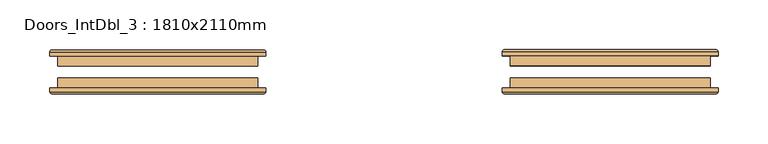
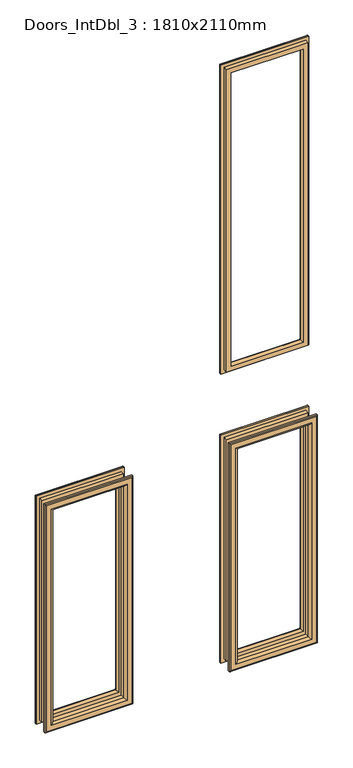
"""IFC4 building model written with IfcOpenShell, lengths in millimetres: door geometry, Doors_IntDbl_3 : 1810x2110mm."""

from ifc_helpers import new_model, si_unit, frame, origin, place, context, project, spatial, ellipse_curve, source, transform, mapped, element, save
from ifc_brep_helpers import plane_surface, cylinder_surface, advanced_brep


def doors_intdbl_3_1810x2110mm_13513f6f(model_context):
    return source(origin(), model_context, "Body", "AdvancedBrep", [
        advanced_brep(
        [(326.5, -79.6, 1885.0), (326.5, -79.6, 1100.0), (326.5, -69.6, 1100.0), (326.5, -69.6, 1885.0), (314.5, -68.6, 1873.0), (314.5, -68.6, 1112.0), (314.5, -79.6, 1112.0), (314.5, -79.6, 1873.0), (319.5, -63.6, 1878.0), (319.5, -63.6, 1107.0), (334.5, -65.6, 1893.0), (334.5, -65.6, 1092.0), (332.5, -63.6, 1094.0), (332.5, -63.6, 1891.0), (334.5, -69.6, 1893.0), (334.5, -69.6, 1092.0), (126.5, -79.6, 1100.0), (126.5, -69.6, 1100.0), (138.5, -68.6, 1112.0), (138.5, -79.6, 1112.0), (133.5, -63.6, 1107.0), (118.5, -65.6, 1092.0), (120.5, -63.6, 1094.0), (118.5, -69.6, 1092.0), (126.5, -79.6, 1885.0), (126.5, -69.6, 1885.0), (138.5, -68.6, 1873.0), (138.5, -79.6, 1873.0), (133.5, -63.6, 1878.0), (118.5, -65.6, 1893.0), (120.5, -63.6, 1891.0), (118.5, -69.6, 1893.0)],
        [
            (0, 1),
            (1, 2),
            (2, 3),
            (3, 0),
            (4, 5),
            (5, 6),
            (6, 7),
            (7, 4),
            (8, 9),
            (9, 5, ellipse_curve(frame((319.5, -68.6, 1107.0), z_axis=(0.7071067811865475, 0.0, 0.7071067811865475), x_axis=(-0.7071067811865474, 0.0, 0.7071067811865476)), 7.0710678, 5.0)),
            (4, 8, ellipse_curve(frame((319.5, -68.6, 1878.0), z_axis=(0.7071067811865475, 0.0, -0.7071067811865475), x_axis=(0.7071067811865474, 0.0, 0.7071067811865476)), 7.0710678, 5.0)),
            (10, 11),
            (11, 12, ellipse_curve(frame((332.5, -65.6, 1094.0), z_axis=(0.7071067811865475, 0.0, 0.7071067811865475), x_axis=(-0.7071067811865474, 0.0, 0.7071067811865476)), 2.8284271, 2.0)),
            (12, 13),
            (13, 10, ellipse_curve(frame((332.5, -65.6, 1891.0), z_axis=(0.7071067811865475, 0.0, -0.7071067811865475), x_axis=(0.7071067811865474, 0.0, 0.7071067811865476)), 2.8284271, 2.0)),
            (14, 15),
            (15, 11),
            (10, 14),
            (1, 16),
            (16, 17),
            (17, 2),
            (5, 18),
            (18, 19),
            (19, 6),
            (9, 20),
            (20, 18, ellipse_curve(frame((133.5, -68.6, 1107.0), z_axis=(0.7071067811865475, 0.0, -0.7071067811865475), x_axis=(0.7071067811865476, 0.0, 0.7071067811865474)), 7.0710678, 5.0)),
            (11, 21),
            (21, 22, ellipse_curve(frame((120.5, -65.6, 1094.0), z_axis=(0.7071067811865475, 0.0, -0.7071067811865475), x_axis=(0.7071067811865476, 0.0, 0.7071067811865474)), 2.8284271, 2.0)),
            (22, 12),
            (15, 23),
            (23, 21),
            (16, 24),
            (24, 25),
            (25, 17),
            (18, 26),
            (26, 27),
            (27, 19),
            (20, 28),
            (28, 26, ellipse_curve(frame((133.5, -68.6, 1878.0), z_axis=(-0.7071067811865475, 0.0, -0.7071067811865475), x_axis=(0.7071067811865474, 0.0, -0.7071067811865476)), 7.0710678, 5.0)),
            (21, 29),
            (29, 30, ellipse_curve(frame((120.5, -65.6, 1891.0), z_axis=(-0.7071067811865475, 0.0, -0.7071067811865475), x_axis=(0.7071067811865474, 0.0, -0.7071067811865476)), 2.8284271, 2.0)),
            (30, 22),
            (23, 31),
            (31, 29),
            (14, 31),
            (25, 3),
            (24, 0),
            (27, 7),
            (26, 4),
            (28, 8),
            (30, 13),
            (29, 10),
        ],
        [
            plane_surface(frame((326.5, -69.6, 1885.0), z_axis=(1.0, 0.0, 0.0), x_axis=(0.0, 0.0, -1.0))),
            plane_surface(frame((314.5, -79.6, 1873.0), z_axis=(-1.0, 0.0, 0.0), x_axis=(0.0, 0.0, -1.0))),
            cylinder_surface(frame((319.5, -68.6, 1885.0), z_axis=(0.0, 0.0, 1.0), x_axis=(1.0, 0.0, 0.0)), 5.0),
            cylinder_surface(frame((332.5, -65.6, 1885.0), z_axis=(0.0, 0.0, 1.0), x_axis=(1.0, 0.0, 0.0)), 2.0),
            plane_surface(frame((334.5, -65.6, 1893.0), z_axis=(1.0, 0.0, 0.0), x_axis=(0.0, 0.0, -1.0))),
            plane_surface(frame((326.5, -69.6, 1100.0), z_axis=(0.0, 0.0, -1.0), x_axis=(-1.0, 0.0, 0.0))),
            plane_surface(frame((314.5, -79.6, 1112.0), z_axis=(0.0, 0.0, 1.0), x_axis=(-1.0, 0.0, 0.0))),
            cylinder_surface(frame((326.5, -68.6, 1107.0), z_axis=(1.0, 0.0, 0.0), x_axis=(0.0, 0.0, -1.0)), 5.0),
            cylinder_surface(frame((326.5, -65.6, 1094.0), z_axis=(1.0, 0.0, 0.0), x_axis=(0.0, 0.0, -1.0)), 2.0),
            plane_surface(frame((334.5, -65.6, 1092.0), z_axis=(0.0, 0.0, -1.0), x_axis=(-1.0, 0.0, 0.0))),
            plane_surface(frame((126.5, -69.6, 1100.0), z_axis=(-1.0, 0.0, 0.0), x_axis=(0.0, 0.0, 1.0))),
            plane_surface(frame((138.5, -79.6, 1112.0), z_axis=(1.0, 0.0, 0.0), x_axis=(0.0, 0.0, 1.0))),
            cylinder_surface(frame((133.5, -68.6, 1100.0), z_axis=(0.0, 0.0, -1.0), x_axis=(-1.0, 0.0, 0.0)), 5.0),
            cylinder_surface(frame((120.5, -65.6, 1100.0), z_axis=(0.0, 0.0, -1.0), x_axis=(-1.0, 0.0, 0.0)), 2.0),
            plane_surface(frame((118.5, -65.6, 1092.0), z_axis=(-1.0, 0.0, 0.0), x_axis=(0.0, 0.0, 1.0))),
            plane_surface(frame((118.5, -69.6, 1893.0), z_axis=(0.0, -1.0, 0.0), x_axis=(1.0, 0.0, 0.0))),
            plane_surface(frame((126.5, -69.6, 1885.0), z_axis=(0.0, 0.0, 1.0), x_axis=(1.0, 0.0, 0.0))),
            plane_surface(frame((126.5, -79.6, 1885.0), z_axis=(0.0, -1.0, 0.0), x_axis=(1.0, 0.0, 0.0))),
            plane_surface(frame((138.5, -79.6, 1873.0), z_axis=(0.0, 0.0, -1.0), x_axis=(1.0, 0.0, 0.0))),
            cylinder_surface(frame((126.5, -68.6, 1878.0), z_axis=(-1.0, 0.0, 0.0), x_axis=(0.0, 0.0, 1.0)), 5.0),
            plane_surface(frame((133.5, -63.6, 1878.0), z_axis=(0.0, 1.0, 0.0), x_axis=(1.0, 0.0, 0.0))),
            cylinder_surface(frame((126.5, -65.6, 1891.0), z_axis=(-1.0, 0.0, 0.0), x_axis=(0.0, 0.0, 1.0)), 2.0),
            plane_surface(frame((118.5, -65.6, 1893.0), z_axis=(0.0, 0.0, 1.0), x_axis=(1.0, 0.0, 0.0))),
        ],
        [
            (0, [[1, 2, 3, 4]]),
            (1, [[5, 6, 7, 8]]),
            (2, [[9, 10, -5, 11]]),
            (3, [[12, 13, 14, 15]]),
            (4, [[16, 17, -12, 18]]),
            (5, [[19, 20, 21, -2]]),
            (6, [[22, 23, 24, -6]]),
            (7, [[25, 26, -22, -10]]),
            (8, [[27, 28, 29, -13]]),
            (9, [[30, 31, -27, -17]]),
            (10, [[32, 33, 34, -20]]),
            (11, [[35, 36, 37, -23]]),
            (12, [[38, 39, -35, -26]]),
            (13, [[40, 41, 42, -28]]),
            (14, [[43, 44, -40, -31]]),
            (15, [[-16, 45, -43, -30], [-3, -21, -34, 46]]),
            (16, [[47, -4, -46, -33]]),
            (17, [[-1, -47, -32, -19], [-7, -24, -37, 48]]),
            (18, [[49, -8, -48, -36]]),
            (19, [[50, -11, -49, -39]]),
            (20, [[-14, -29, -42, 51], [-9, -50, -38, -25]]),
            (21, [[52, -15, -51, -41]]),
            (22, [[-45, -18, -52, -44]]),
        ],
    ),
        advanced_brep(
        [(118.5, -105.6, 342.0), (118.5, -105.6, 933.0), (118.5, -101.6, 933.0), (118.5, -101.6, 342.0), (120.5, -107.6, 344.0), (120.5, -107.6, 931.0), (138.5, -102.6, 362.0), (138.5, -102.6, 913.0), (133.5, -107.6, 918.0), (133.5, -107.6, 357.0), (138.5, -91.6, 362.0), (138.5, -91.6, 913.0), (126.5, -101.6, 350.0), (126.5, -101.6, 925.0), (126.5, -91.6, 925.0), (126.5, -91.6, 350.0), (334.5, -105.6, 933.0), (334.5, -101.6, 933.0), (332.5, -107.6, 931.0), (314.5, -102.6, 913.0), (319.5, -107.6, 918.0), (314.5, -91.6, 913.0), (326.5, -101.6, 925.0), (326.5, -91.6, 925.0), (334.5, -105.6, 342.0), (334.5, -101.6, 342.0), (332.5, -107.6, 344.0), (314.5, -102.6, 362.0), (319.5, -107.6, 357.0), (314.5, -91.6, 362.0), (326.5, -101.6, 350.0), (326.5, -91.6, 350.0)],
        [
            (0, 1),
            (1, 2),
            (2, 3),
            (3, 0),
            (4, 5),
            (5, 1, ellipse_curve(frame((120.5, -105.6, 931.0), z_axis=(-0.7071067811865475, 0.0, -0.7071067811865475), x_axis=(0.7071067811865474, 0.0, -0.7071067811865476)), 2.8284271, 2.0)),
            (0, 4, ellipse_curve(frame((120.5, -105.6, 344.0), z_axis=(-0.7071067811865475, 0.0, 0.7071067811865475), x_axis=(-0.7071067811865474, 0.0, -0.7071067811865476)), 2.8284271, 2.0)),
            (6, 7),
            (7, 8, ellipse_curve(frame((133.5, -102.6, 918.0), z_axis=(-0.7071067811865475, 0.0, -0.7071067811865475), x_axis=(0.7071067811865474, 0.0, -0.7071067811865476)), 7.0710678, 5.0)),
            (8, 9),
            (9, 6, ellipse_curve(frame((133.5, -102.6, 357.0), z_axis=(-0.7071067811865475, 0.0, 0.7071067811865475), x_axis=(-0.7071067811865474, 0.0, -0.7071067811865476)), 7.0710678, 5.0)),
            (10, 11),
            (11, 7),
            (6, 10),
            (12, 13),
            (13, 14),
            (14, 15),
            (15, 12),
            (1, 16),
            (16, 17),
            (17, 2),
            (5, 18),
            (18, 16, ellipse_curve(frame((332.5, -105.6, 931.0), z_axis=(-0.7071067811865475, 0.0, 0.7071067811865475), x_axis=(-0.7071067811865476, 0.0, -0.7071067811865474)), 2.8284271, 2.0)),
            (7, 19),
            (19, 20, ellipse_curve(frame((319.5, -102.6, 918.0), z_axis=(-0.7071067811865475, 0.0, 0.7071067811865475), x_axis=(-0.7071067811865476, 0.0, -0.7071067811865474)), 7.0710678, 5.0)),
            (20, 8),
            (11, 21),
            (21, 19),
            (13, 22),
            (22, 23),
            (23, 14),
            (16, 24),
            (24, 25),
            (25, 17),
            (18, 26),
            (26, 24, ellipse_curve(frame((332.5, -105.6, 344.0), z_axis=(0.7071067811865475, 0.0, 0.7071067811865475), x_axis=(-0.7071067811865474, 0.0, 0.7071067811865476)), 2.8284271, 2.0)),
            (19, 27),
            (27, 28, ellipse_curve(frame((319.5, -102.6, 357.0), z_axis=(0.7071067811865475, 0.0, 0.7071067811865475), x_axis=(-0.7071067811865474, 0.0, 0.7071067811865476)), 7.0710678, 5.0)),
            (28, 20),
            (21, 29),
            (29, 27),
            (22, 30),
            (30, 31),
            (31, 23),
            (24, 0),
            (3, 25),
            (26, 4),
            (28, 9),
            (27, 6),
            (29, 10),
            (31, 15),
            (30, 12),
        ],
        [
            plane_surface(frame((118.5, -101.6, 342.0), z_axis=(-1.0, 0.0, 0.0), x_axis=(0.0, 0.0, 1.0))),
            cylinder_surface(frame((120.5, -105.6, 350.0), z_axis=(0.0, 0.0, -1.0), x_axis=(-1.0, 0.0, 0.0)), 2.0),
            cylinder_surface(frame((133.5, -102.6, 350.0), z_axis=(0.0, 0.0, -1.0), x_axis=(-1.0, 0.0, 0.0)), 5.0),
            plane_surface(frame((138.5, -102.6, 362.0), z_axis=(1.0, 0.0, 0.0), x_axis=(0.0, 0.0, 1.0))),
            plane_surface(frame((126.5, -91.6, 350.0), z_axis=(-1.0, 0.0, 0.0), x_axis=(0.0, 0.0, 1.0))),
            plane_surface(frame((118.5, -101.6, 933.0), z_axis=(0.0, 0.0, 1.0), x_axis=(1.0, 0.0, 0.0))),
            cylinder_surface(frame((126.5, -105.6, 931.0), z_axis=(-1.0, 0.0, 0.0), x_axis=(0.0, 0.0, 1.0)), 2.0),
            cylinder_surface(frame((126.5, -102.6, 918.0), z_axis=(-1.0, 0.0, 0.0), x_axis=(0.0, 0.0, 1.0)), 5.0),
            plane_surface(frame((138.5, -102.6, 913.0), z_axis=(0.0, 0.0, -1.0), x_axis=(1.0, 0.0, 0.0))),
            plane_surface(frame((126.5, -91.6, 925.0), z_axis=(0.0, 0.0, 1.0), x_axis=(1.0, 0.0, 0.0))),
            plane_surface(frame((334.5, -101.6, 933.0), z_axis=(1.0, 0.0, 0.0), x_axis=(0.0, 0.0, -1.0))),
            cylinder_surface(frame((332.5, -105.6, 925.0), z_axis=(0.0, 0.0, 1.0), x_axis=(1.0, 0.0, 0.0)), 2.0),
            cylinder_surface(frame((319.5, -102.6, 925.0), z_axis=(0.0, 0.0, 1.0), x_axis=(1.0, 0.0, 0.0)), 5.0),
            plane_surface(frame((314.5, -102.6, 913.0), z_axis=(-1.0, 0.0, 0.0), x_axis=(0.0, 0.0, -1.0))),
            plane_surface(frame((326.5, -91.6, 925.0), z_axis=(1.0, 0.0, 0.0), x_axis=(0.0, 0.0, -1.0))),
            plane_surface(frame((334.5, -101.6, 342.0), z_axis=(0.0, 0.0, -1.0), x_axis=(-1.0, 0.0, 0.0))),
            cylinder_surface(frame((326.5, -105.6, 344.0), z_axis=(1.0, 0.0, 0.0), x_axis=(0.0, 0.0, -1.0)), 2.0),
            plane_surface(frame((332.5, -107.6, 344.0), z_axis=(0.0, -1.0, 0.0), x_axis=(-1.0, 0.0, 0.0))),
            cylinder_surface(frame((326.5, -102.6, 357.0), z_axis=(1.0, 0.0, 0.0), x_axis=(0.0, 0.0, -1.0)), 5.0),
            plane_surface(frame((314.5, -102.6, 362.0), z_axis=(0.0, 0.0, 1.0), x_axis=(-1.0, 0.0, 0.0))),
            plane_surface(frame((314.5, -91.6, 362.0), z_axis=(0.0, 1.0, 0.0), x_axis=(-1.0, 0.0, 0.0))),
            plane_surface(frame((326.5, -91.6, 350.0), z_axis=(0.0, 0.0, -1.0), x_axis=(-1.0, 0.0, 0.0))),
            plane_surface(frame((326.5, -101.6, 350.0), z_axis=(0.0, 1.0, 0.0), x_axis=(-1.0, 0.0, 0.0))),
        ],
        [
            (0, [[1, 2, 3, 4]]),
            (1, [[5, 6, -1, 7]]),
            (2, [[8, 9, 10, 11]]),
            (3, [[12, 13, -8, 14]]),
            (4, [[15, 16, 17, 18]]),
            (5, [[19, 20, 21, -2]]),
            (6, [[22, 23, -19, -6]]),
            (7, [[24, 25, 26, -9]]),
            (8, [[27, 28, -24, -13]]),
            (9, [[29, 30, 31, -16]]),
            (10, [[32, 33, 34, -20]]),
            (11, [[35, 36, -32, -23]]),
            (12, [[37, 38, 39, -25]]),
            (13, [[40, 41, -37, -28]]),
            (14, [[42, 43, 44, -30]]),
            (15, [[45, -4, 46, -33]]),
            (16, [[47, -7, -45, -36]]),
            (17, [[-5, -47, -35, -22], [-10, -26, -39, 48]]),
            (18, [[49, -11, -48, -38]]),
            (19, [[50, -14, -49, -41]]),
            (20, [[-17, -31, -44, 51], [-12, -50, -40, -27]]),
            (21, [[52, -18, -51, -43]]),
            (22, [[-3, -21, -34, -46], [-15, -52, -42, -29]]),
        ],
    ),
        advanced_brep(
        [(-334.5, -105.6, 342.0), (-334.5, -105.6, 933.0), (-334.5, -101.6, 933.0), (-334.5, -101.6, 342.0), (-332.5, -107.6, 344.0), (-332.5, -107.6, 931.0), (-314.5, -102.6, 362.0), (-314.5, -102.6, 913.0), (-319.5, -107.6, 918.0), (-319.5, -107.6, 357.0), (-314.5, -91.6, 362.0), (-314.5, -91.6, 913.0), (-326.5, -101.6, 350.0), (-326.5, -101.6, 925.0), (-326.5, -91.6, 925.0), (-326.5, -91.6, 350.0), (-118.5, -105.6, 933.0), (-118.5, -101.6, 933.0), (-120.5, -107.6, 931.0), (-138.5, -102.6, 913.0), (-133.5, -107.6, 918.0), (-138.5, -91.6, 913.0), (-126.5, -101.6, 925.0), (-126.5, -91.6, 925.0), (-118.5, -105.6, 342.0), (-118.5, -101.6, 342.0), (-120.5, -107.6, 344.0), (-138.5, -102.6, 362.0), (-133.5, -107.6, 357.0), (-138.5, -91.6, 362.0), (-126.5, -101.6, 350.0), (-126.5, -91.6, 350.0)],
        [
            (0, 1),
            (1, 2),
            (2, 3),
            (3, 0),
            (4, 5),
            (5, 1, ellipse_curve(frame((-332.5, -105.6, 931.0), z_axis=(-0.7071067811865475, 0.0, -0.7071067811865475), x_axis=(0.7071067811865474, 0.0, -0.7071067811865476)), 2.8284271, 2.0)),
            (0, 4, ellipse_curve(frame((-332.5, -105.6, 344.0), z_axis=(-0.7071067811865475, 0.0, 0.7071067811865475), x_axis=(-0.7071067811865474, 0.0, -0.7071067811865476)), 2.8284271, 2.0)),
            (6, 7),
            (7, 8, ellipse_curve(frame((-319.5, -102.6, 918.0), z_axis=(-0.7071067811865475, 0.0, -0.7071067811865475), x_axis=(0.7071067811865474, 0.0, -0.7071067811865476)), 7.0710678, 5.0)),
            (8, 9),
            (9, 6, ellipse_curve(frame((-319.5, -102.6, 357.0), z_axis=(-0.7071067811865475, 0.0, 0.7071067811865475), x_axis=(-0.7071067811865474, 0.0, -0.7071067811865476)), 7.0710678, 5.0)),
            (10, 11),
            (11, 7),
            (6, 10),
            (12, 13),
            (13, 14),
            (14, 15),
            (15, 12),
            (1, 16),
            (16, 17),
            (17, 2),
            (5, 18),
            (18, 16, ellipse_curve(frame((-120.5, -105.6, 931.0), z_axis=(-0.7071067811865475, 0.0, 0.7071067811865475), x_axis=(-0.7071067811865476, 0.0, -0.7071067811865474)), 2.8284271, 2.0)),
            (7, 19),
            (19, 20, ellipse_curve(frame((-133.5, -102.6, 918.0), z_axis=(-0.7071067811865475, 0.0, 0.7071067811865475), x_axis=(-0.7071067811865476, 0.0, -0.7071067811865474)), 7.0710678, 5.0)),
            (20, 8),
            (11, 21),
            (21, 19),
            (13, 22),
            (22, 23),
            (23, 14),
            (16, 24),
            (24, 25),
            (25, 17),
            (18, 26),
            (26, 24, ellipse_curve(frame((-120.5, -105.6, 344.0), z_axis=(0.7071067811865475, 0.0, 0.7071067811865475), x_axis=(-0.7071067811865474, 0.0, 0.7071067811865476)), 2.8284271, 2.0)),
            (19, 27),
            (27, 28, ellipse_curve(frame((-133.5, -102.6, 357.0), z_axis=(0.7071067811865475, 0.0, 0.7071067811865475), x_axis=(-0.7071067811865474, 0.0, 0.7071067811865476)), 7.0710678, 5.0)),
            (28, 20),
            (21, 29),
            (29, 27),
            (22, 30),
            (30, 31),
            (31, 23),
            (24, 0),
            (3, 25),
            (26, 4),
            (28, 9),
            (27, 6),
            (29, 10),
            (31, 15),
            (30, 12),
        ],
        [
            plane_surface(frame((-334.5, -101.6, 342.0), z_axis=(-1.0, 0.0, 0.0), x_axis=(0.0, 0.0, 1.0))),
            cylinder_surface(frame((-332.5, -105.6, 350.0), z_axis=(0.0, 0.0, -1.0), x_axis=(-1.0, 0.0, 0.0)), 2.0),
            cylinder_surface(frame((-319.5, -102.6, 350.0), z_axis=(0.0, 0.0, -1.0), x_axis=(-1.0, 0.0, 0.0)), 5.0),
            plane_surface(frame((-314.5, -102.6, 362.0), z_axis=(1.0, 0.0, 0.0), x_axis=(0.0, 0.0, 1.0))),
            plane_surface(frame((-326.5, -91.6, 350.0), z_axis=(-1.0, 0.0, 0.0), x_axis=(0.0, 0.0, 1.0))),
            plane_surface(frame((-334.5, -101.6, 933.0), z_axis=(0.0, 0.0, 1.0), x_axis=(1.0, 0.0, 0.0))),
            cylinder_surface(frame((-326.5, -105.6, 931.0), z_axis=(-1.0, 0.0, 0.0), x_axis=(0.0, 0.0, 1.0)), 2.0),
            cylinder_surface(frame((-326.5, -102.6, 918.0), z_axis=(-1.0, 0.0, 0.0), x_axis=(0.0, 0.0, 1.0)), 5.0),
            plane_surface(frame((-314.5, -102.6, 913.0), z_axis=(0.0, 0.0, -1.0), x_axis=(1.0, 0.0, 0.0))),
            plane_surface(frame((-326.5, -91.6, 925.0), z_axis=(0.0, 0.0, 1.0), x_axis=(1.0, 0.0, 0.0))),
            plane_surface(frame((-118.5, -101.6, 933.0), z_axis=(1.0, 0.0, 0.0), x_axis=(0.0, 0.0, -1.0))),
            cylinder_surface(frame((-120.5, -105.6, 925.0), z_axis=(0.0, 0.0, 1.0), x_axis=(1.0, 0.0, 0.0)), 2.0),
            cylinder_surface(frame((-133.5, -102.6, 925.0), z_axis=(0.0, 0.0, 1.0), x_axis=(1.0, 0.0, 0.0)), 5.0),
            plane_surface(frame((-138.5, -102.6, 913.0), z_axis=(-1.0, 0.0, 0.0), x_axis=(0.0, 0.0, -1.0))),
            plane_surface(frame((-126.5, -91.6, 925.0), z_axis=(1.0, 0.0, 0.0), x_axis=(0.0, 0.0, -1.0))),
            plane_surface(frame((-118.5, -101.6, 342.0), z_axis=(0.0, 0.0, -1.0), x_axis=(-1.0, 0.0, 0.0))),
            cylinder_surface(frame((-126.5, -105.6, 344.0), z_axis=(1.0, 0.0, 0.0), x_axis=(0.0, 0.0, -1.0)), 2.0),
            plane_surface(frame((-120.5, -107.6, 344.0), z_axis=(0.0, -1.0, 0.0), x_axis=(-1.0, 0.0, 0.0))),
            cylinder_surface(frame((-126.5, -102.6, 357.0), z_axis=(1.0, 0.0, 0.0), x_axis=(0.0, 0.0, -1.0)), 5.0),
            plane_surface(frame((-138.5, -102.6, 362.0), z_axis=(0.0, 0.0, 1.0), x_axis=(-1.0, 0.0, 0.0))),
            plane_surface(frame((-138.5, -91.6, 362.0), z_axis=(0.0, 1.0, 0.0), x_axis=(-1.0, 0.0, 0.0))),
            plane_surface(frame((-126.5, -91.6, 350.0), z_axis=(0.0, 0.0, -1.0), x_axis=(-1.0, 0.0, 0.0))),
            plane_surface(frame((-126.5, -101.6, 350.0), z_axis=(0.0, 1.0, 0.0), x_axis=(-1.0, 0.0, 0.0))),
        ],
        [
            (0, [[1, 2, 3, 4]]),
            (1, [[5, 6, -1, 7]]),
            (2, [[8, 9, 10, 11]]),
            (3, [[12, 13, -8, 14]]),
            (4, [[15, 16, 17, 18]]),
            (5, [[19, 20, 21, -2]]),
            (6, [[22, 23, -19, -6]]),
            (7, [[24, 25, 26, -9]]),
            (8, [[27, 28, -24, -13]]),
            (9, [[29, 30, 31, -16]]),
            (10, [[32, 33, 34, -20]]),
            (11, [[35, 36, -32, -23]]),
            (12, [[37, 38, 39, -25]]),
            (13, [[40, 41, -37, -28]]),
            (14, [[42, 43, 44, -30]]),
            (15, [[45, -4, 46, -33]]),
            (16, [[47, -7, -45, -36]]),
            (17, [[-5, -47, -35, -22], [-10, -26, -39, 48]]),
            (18, [[49, -11, -48, -38]]),
            (19, [[50, -14, -49, -41]]),
            (20, [[-17, -31, -44, 51], [-12, -50, -40, -27]]),
            (21, [[52, -18, -51, -43]]),
            (22, [[-3, -21, -34, -46], [-15, -52, -42, -29]]),
        ],
    ),
        advanced_brep(
        [(-126.5, -79.6, 925.0), (-126.5, -79.6, 350.0), (-126.5, -69.6, 350.0), (-126.5, -69.6, 925.0), (-138.5, -68.6, 913.0), (-138.5, -68.6, 362.0), (-138.5, -79.6, 362.0), (-138.5, -79.6, 913.0), (-133.5, -63.6, 918.0), (-133.5, -63.6, 357.0), (-118.5, -65.6, 933.0), (-118.5, -65.6, 342.0), (-120.5, -63.6, 344.0), (-120.5, -63.6, 931.0), (-118.5, -69.6, 933.0), (-118.5, -69.6, 342.0), (-326.5, -79.6, 350.0), (-326.5, -69.6, 350.0), (-314.5, -68.6, 362.0), (-314.5, -79.6, 362.0), (-319.5, -63.6, 357.0), (-334.5, -65.6, 342.0), (-332.5, -63.6, 344.0), (-334.5, -69.6, 342.0), (-326.5, -79.6, 925.0), (-326.5, -69.6, 925.0), (-314.5, -68.6, 913.0), (-314.5, -79.6, 913.0), (-319.5, -63.6, 918.0), (-334.5, -65.6, 933.0), (-332.5, -63.6, 931.0), (-334.5, -69.6, 933.0)],
        [
            (0, 1),
            (1, 2),
            (2, 3),
            (3, 0),
            (4, 5),
            (5, 6),
            (6, 7),
            (7, 4),
            (8, 9),
            (9, 5, ellipse_curve(frame((-133.5, -68.6, 357.0), z_axis=(0.7071067811865475, 0.0, 0.7071067811865475), x_axis=(-0.7071067811865474, 0.0, 0.7071067811865476)), 7.0710678, 5.0)),
            (4, 8, ellipse_curve(frame((-133.5, -68.6, 918.0), z_axis=(0.7071067811865475, 0.0, -0.7071067811865475), x_axis=(0.7071067811865474, 0.0, 0.7071067811865476)), 7.0710678, 5.0)),
            (10, 11),
            (11, 12, ellipse_curve(frame((-120.5, -65.6, 344.0), z_axis=(0.7071067811865475, 0.0, 0.7071067811865475), x_axis=(-0.7071067811865474, 0.0, 0.7071067811865476)), 2.8284271, 2.0)),
            (12, 13),
            (13, 10, ellipse_curve(frame((-120.5, -65.6, 931.0), z_axis=(0.7071067811865475, 0.0, -0.7071067811865475), x_axis=(0.7071067811865474, 0.0, 0.7071067811865476)), 2.8284271, 2.0)),
            (14, 15),
            (15, 11),
            (10, 14),
            (1, 16),
            (16, 17),
            (17, 2),
            (5, 18),
            (18, 19),
            (19, 6),
            (9, 20),
            (20, 18, ellipse_curve(frame((-319.5, -68.6, 357.0), z_axis=(0.7071067811865475, 0.0, -0.7071067811865475), x_axis=(0.7071067811865476, 0.0, 0.7071067811865474)), 7.0710678, 5.0)),
            (11, 21),
            (21, 22, ellipse_curve(frame((-332.5, -65.6, 344.0), z_axis=(0.7071067811865475, 0.0, -0.7071067811865475), x_axis=(0.7071067811865476, 0.0, 0.7071067811865474)), 2.8284271, 2.0)),
            (22, 12),
            (15, 23),
            (23, 21),
            (16, 24),
            (24, 25),
            (25, 17),
            (18, 26),
            (26, 27),
            (27, 19),
            (20, 28),
            (28, 26, ellipse_curve(frame((-319.5, -68.6, 918.0), z_axis=(-0.7071067811865475, 0.0, -0.7071067811865475), x_axis=(0.7071067811865474, 0.0, -0.7071067811865476)), 7.0710678, 5.0)),
            (21, 29),
            (29, 30, ellipse_curve(frame((-332.5, -65.6, 931.0), z_axis=(-0.7071067811865475, 0.0, -0.7071067811865475), x_axis=(0.7071067811865474, 0.0, -0.7071067811865476)), 2.8284271, 2.0)),
            (30, 22),
            (23, 31),
            (31, 29),
            (14, 31),
            (25, 3),
            (24, 0),
            (27, 7),
            (26, 4),
            (28, 8),
            (30, 13),
            (29, 10),
        ],
        [
            plane_surface(frame((-126.5, -69.6, 925.0), z_axis=(1.0, 0.0, 0.0), x_axis=(0.0, 0.0, -1.0))),
            plane_surface(frame((-138.5, -79.6, 913.0), z_axis=(-1.0, 0.0, 0.0), x_axis=(0.0, 0.0, -1.0))),
            cylinder_surface(frame((-133.5, -68.6, 925.0), z_axis=(0.0, 0.0, 1.0), x_axis=(1.0, 0.0, 0.0)), 5.0),
            cylinder_surface(frame((-120.5, -65.6, 925.0), z_axis=(0.0, 0.0, 1.0), x_axis=(1.0, 0.0, 0.0)), 2.0),
            plane_surface(frame((-118.5, -65.6, 933.0), z_axis=(1.0, 0.0, 0.0), x_axis=(0.0, 0.0, -1.0))),
            plane_surface(frame((-126.5, -69.6, 350.0), z_axis=(0.0, 0.0, -1.0), x_axis=(-1.0, 0.0, 0.0))),
            plane_surface(frame((-138.5, -79.6, 362.0), z_axis=(0.0, 0.0, 1.0), x_axis=(-1.0, 0.0, 0.0))),
            cylinder_surface(frame((-126.5, -68.6, 357.0), z_axis=(1.0, 0.0, 0.0), x_axis=(0.0, 0.0, -1.0)), 5.0),
            cylinder_surface(frame((-126.5, -65.6, 344.0), z_axis=(1.0, 0.0, 0.0), x_axis=(0.0, 0.0, -1.0)), 2.0),
            plane_surface(frame((-118.5, -65.6, 342.0), z_axis=(0.0, 0.0, -1.0), x_axis=(-1.0, 0.0, 0.0))),
            plane_surface(frame((-326.5, -69.6, 350.0), z_axis=(-1.0, 0.0, 0.0), x_axis=(0.0, 0.0, 1.0))),
            plane_surface(frame((-314.5, -79.6, 362.0), z_axis=(1.0, 0.0, 0.0), x_axis=(0.0, 0.0, 1.0))),
            cylinder_surface(frame((-319.5, -68.6, 350.0), z_axis=(0.0, 0.0, -1.0), x_axis=(-1.0, 0.0, 0.0)), 5.0),
            cylinder_surface(frame((-332.5, -65.6, 350.0), z_axis=(0.0, 0.0, -1.0), x_axis=(-1.0, 0.0, 0.0)), 2.0),
            plane_surface(frame((-334.5, -65.6, 342.0), z_axis=(-1.0, 0.0, 0.0), x_axis=(0.0, 0.0, 1.0))),
            plane_surface(frame((-334.5, -69.6, 933.0), z_axis=(0.0, -1.0, 0.0), x_axis=(1.0, 0.0, 0.0))),
            plane_surface(frame((-326.5, -69.6, 925.0), z_axis=(0.0, 0.0, 1.0), x_axis=(1.0, 0.0, 0.0))),
            plane_surface(frame((-326.5, -79.6, 925.0), z_axis=(0.0, -1.0, 0.0), x_axis=(1.0, 0.0, 0.0))),
            plane_surface(frame((-314.5, -79.6, 913.0), z_axis=(0.0, 0.0, -1.0), x_axis=(1.0, 0.0, 0.0))),
            cylinder_surface(frame((-326.5, -68.6, 918.0), z_axis=(-1.0, 0.0, 0.0), x_axis=(0.0, 0.0, 1.0)), 5.0),
            plane_surface(frame((-319.5, -63.6, 918.0), z_axis=(0.0, 1.0, 0.0), x_axis=(1.0, 0.0, 0.0))),
            cylinder_surface(frame((-326.5, -65.6, 931.0), z_axis=(-1.0, 0.0, 0.0), x_axis=(0.0, 0.0, 1.0)), 2.0),
            plane_surface(frame((-334.5, -65.6, 933.0), z_axis=(0.0, 0.0, 1.0), x_axis=(1.0, 0.0, 0.0))),
        ],
        [
            (0, [[1, 2, 3, 4]]),
            (1, [[5, 6, 7, 8]]),
            (2, [[9, 10, -5, 11]]),
            (3, [[12, 13, 14, 15]]),
            (4, [[16, 17, -12, 18]]),
            (5, [[19, 20, 21, -2]]),
            (6, [[22, 23, 24, -6]]),
            (7, [[25, 26, -22, -10]]),
            (8, [[27, 28, 29, -13]]),
            (9, [[30, 31, -27, -17]]),
            (10, [[32, 33, 34, -20]]),
            (11, [[35, 36, 37, -23]]),
            (12, [[38, 39, -35, -26]]),
            (13, [[40, 41, 42, -28]]),
            (14, [[43, 44, -40, -31]]),
            (15, [[-16, 45, -43, -30], [-3, -21, -34, 46]]),
            (16, [[47, -4, -46, -33]]),
            (17, [[-1, -47, -32, -19], [-7, -24, -37, 48]]),
            (18, [[49, -8, -48, -36]]),
            (19, [[50, -11, -49, -39]]),
            (20, [[-14, -29, -42, 51], [-9, -50, -38, -25]]),
            (21, [[52, -15, -51, -41]]),
            (22, [[-45, -18, -52, -44]]),
        ],
    ),
        advanced_brep(
        [(334.5, -65.6, 342.0), (334.5, -65.6, 933.0), (334.5, -69.6, 933.0), (334.5, -69.6, 342.0), (332.5, -63.6, 344.0), (332.5, -63.6, 931.0), (314.5, -68.6, 362.0), (314.5, -68.6, 913.0), (319.5, -63.6, 918.0), (319.5, -63.6, 357.0), (314.5, -79.6, 362.0), (314.5, -79.6, 913.0), (326.5, -69.6, 350.0), (326.5, -69.6, 925.0), (326.5, -79.6, 925.0), (326.5, -79.6, 350.0), (118.5, -65.6, 933.0), (118.5, -69.6, 933.0), (120.5, -63.6, 931.0), (138.5, -68.6, 913.0), (133.5, -63.6, 918.0), (138.5, -79.6, 913.0), (126.5, -69.6, 925.0), (126.5, -79.6, 925.0), (118.5, -65.6, 342.0), (118.5, -69.6, 342.0), (120.5, -63.6, 344.0), (138.5, -68.6, 362.0), (133.5, -63.6, 357.0), (138.5, -79.6, 362.0), (126.5, -69.6, 350.0), (126.5, -79.6, 350.0)],
        [
            (0, 1),
            (1, 2),
            (2, 3),
            (3, 0),
            (4, 5),
            (5, 1, ellipse_curve(frame((332.5, -65.6, 931.0), z_axis=(0.7071067811865475, 0.0, -0.7071067811865475), x_axis=(-0.7071067811865474, 0.0, -0.7071067811865476)), 2.8284271, 2.0)),
            (0, 4, ellipse_curve(frame((332.5, -65.6, 344.0), z_axis=(0.7071067811865475, 0.0, 0.7071067811865475), x_axis=(0.7071067811865474, 0.0, -0.7071067811865476)), 2.8284271, 2.0)),
            (6, 7),
            (7, 8, ellipse_curve(frame((319.5, -68.6, 918.0), z_axis=(0.7071067811865475, 0.0, -0.7071067811865475), x_axis=(-0.7071067811865474, 0.0, -0.7071067811865476)), 7.0710678, 5.0)),
            (8, 9),
            (9, 6, ellipse_curve(frame((319.5, -68.6, 357.0), z_axis=(0.7071067811865475, 0.0, 0.7071067811865475), x_axis=(0.7071067811865474, 0.0, -0.7071067811865476)), 7.0710678, 5.0)),
            (10, 11),
            (11, 7),
            (6, 10),
            (12, 13),
            (13, 14),
            (14, 15),
            (15, 12),
            (1, 16),
            (16, 17),
            (17, 2),
            (5, 18),
            (18, 16, ellipse_curve(frame((120.5, -65.6, 931.0), z_axis=(0.7071067811865475, 0.0, 0.7071067811865475), x_axis=(0.7071067811865476, 0.0, -0.7071067811865474)), 2.8284271, 2.0)),
            (7, 19),
            (19, 20, ellipse_curve(frame((133.5, -68.6, 918.0), z_axis=(0.7071067811865475, 0.0, 0.7071067811865475), x_axis=(0.7071067811865476, 0.0, -0.7071067811865474)), 7.0710678, 5.0)),
            (20, 8),
            (11, 21),
            (21, 19),
            (13, 22),
            (22, 23),
            (23, 14),
            (16, 24),
            (24, 25),
            (25, 17),
            (18, 26),
            (26, 24, ellipse_curve(frame((120.5, -65.6, 344.0), z_axis=(-0.7071067811865475, 0.0, 0.7071067811865475), x_axis=(0.7071067811865474, 0.0, 0.7071067811865476)), 2.8284271, 2.0)),
            (19, 27),
            (27, 28, ellipse_curve(frame((133.5, -68.6, 357.0), z_axis=(-0.7071067811865475, 0.0, 0.7071067811865475), x_axis=(0.7071067811865474, 0.0, 0.7071067811865476)), 7.0710678, 5.0)),
            (28, 20),
            (21, 29),
            (29, 27),
            (22, 30),
            (30, 31),
            (31, 23),
            (24, 0),
            (3, 25),
            (26, 4),
            (28, 9),
            (27, 6),
            (29, 10),
            (31, 15),
            (30, 12),
        ],
        [
            plane_surface(frame((334.5, -69.6, 342.0), z_axis=(1.0, 0.0, 0.0), x_axis=(0.0, 0.0, 1.0))),
            cylinder_surface(frame((332.5, -65.6, 350.0), z_axis=(0.0, 0.0, -1.0), x_axis=(1.0, 0.0, 0.0)), 2.0),
            cylinder_surface(frame((319.5, -68.6, 350.0), z_axis=(0.0, 0.0, -1.0), x_axis=(1.0, 0.0, 0.0)), 5.0),
            plane_surface(frame((314.5, -68.6, 362.0), z_axis=(-1.0, 0.0, 0.0), x_axis=(0.0, 0.0, 1.0))),
            plane_surface(frame((326.5, -79.6, 350.0), z_axis=(1.0, 0.0, 0.0), x_axis=(0.0, 0.0, 1.0))),
            plane_surface(frame((334.5, -69.6, 933.0), z_axis=(0.0, 0.0, 1.0), x_axis=(-1.0, 0.0, 0.0))),
            cylinder_surface(frame((326.5, -65.6, 931.0), z_axis=(1.0, 0.0, 0.0), x_axis=(0.0, 0.0, 1.0)), 2.0),
            cylinder_surface(frame((326.5, -68.6, 918.0), z_axis=(1.0, 0.0, 0.0), x_axis=(0.0, 0.0, 1.0)), 5.0),
            plane_surface(frame((314.5, -68.6, 913.0), z_axis=(0.0, 0.0, -1.0), x_axis=(-1.0, 0.0, 0.0))),
            plane_surface(frame((326.5, -79.6, 925.0), z_axis=(0.0, 0.0, 1.0), x_axis=(-1.0, 0.0, 0.0))),
            plane_surface(frame((118.5, -69.6, 933.0), z_axis=(-1.0, 0.0, 0.0), x_axis=(0.0, 0.0, -1.0))),
            cylinder_surface(frame((120.5, -65.6, 925.0), z_axis=(0.0, 0.0, 1.0), x_axis=(-1.0, 0.0, 0.0)), 2.0),
            cylinder_surface(frame((133.5, -68.6, 925.0), z_axis=(0.0, 0.0, 1.0), x_axis=(-1.0, 0.0, 0.0)), 5.0),
            plane_surface(frame((138.5, -68.6, 913.0), z_axis=(1.0, 0.0, 0.0), x_axis=(0.0, 0.0, -1.0))),
            plane_surface(frame((126.5, -79.6, 925.0), z_axis=(-1.0, 0.0, 0.0), x_axis=(0.0, 0.0, -1.0))),
            plane_surface(frame((118.5, -69.6, 342.0), z_axis=(0.0, 0.0, -1.0), x_axis=(1.0, 0.0, 0.0))),
            cylinder_surface(frame((126.5, -65.6, 344.0), z_axis=(-1.0, 0.0, 0.0), x_axis=(0.0, 0.0, -1.0)), 2.0),
            plane_surface(frame((120.5, -63.6, 344.0), z_axis=(0.0, 1.0, 0.0), x_axis=(1.0, 0.0, 0.0))),
            cylinder_surface(frame((126.5, -68.6, 357.0), z_axis=(-1.0, 0.0, 0.0), x_axis=(0.0, 0.0, -1.0)), 5.0),
            plane_surface(frame((138.5, -68.6, 362.0), z_axis=(0.0, 0.0, 1.0), x_axis=(1.0, 0.0, 0.0))),
            plane_surface(frame((138.5, -79.6, 362.0), z_axis=(0.0, -1.0, 0.0), x_axis=(1.0, 0.0, 0.0))),
            plane_surface(frame((126.5, -79.6, 350.0), z_axis=(0.0, 0.0, -1.0), x_axis=(1.0, 0.0, 0.0))),
            plane_surface(frame((126.5, -69.6, 350.0), z_axis=(0.0, -1.0, 0.0), x_axis=(1.0, 0.0, 0.0))),
        ],
        [
            (0, [[1, 2, 3, 4]]),
            (1, [[5, 6, -1, 7]]),
            (2, [[8, 9, 10, 11]]),
            (3, [[12, 13, -8, 14]]),
            (4, [[15, 16, 17, 18]]),
            (5, [[19, 20, 21, -2]]),
            (6, [[22, 23, -19, -6]]),
            (7, [[24, 25, 26, -9]]),
            (8, [[27, 28, -24, -13]]),
            (9, [[29, 30, 31, -16]]),
            (10, [[32, 33, 34, -20]]),
            (11, [[35, 36, -32, -23]]),
            (12, [[37, 38, 39, -25]]),
            (13, [[40, 41, -37, -28]]),
            (14, [[42, 43, 44, -30]]),
            (15, [[45, -4, 46, -33]]),
            (16, [[47, -7, -45, -36]]),
            (17, [[-5, -47, -35, -22], [-10, -26, -39, 48]]),
            (18, [[49, -11, -48, -38]]),
            (19, [[50, -14, -49, -41]]),
            (20, [[-17, -31, -44, 51], [-12, -50, -40, -27]]),
            (21, [[52, -18, -51, -43]]),
            (22, [[-3, -21, -34, -46], [-15, -52, -42, -29]]),
        ],
    ),
    ])


if __name__ == "__main__":
    model = new_model("IFC4")
    model_context = context("Model", 3, world=origin())
    ifc_project = project(units=[si_unit("LENGTHUNIT", "METRE", prefix="MILLI")], contexts=[model_context])
    site = spatial("IfcSite", under=ifc_project)
    building = spatial("IfcBuilding", under=site)
    placement = place(None, origin())
    doors_intdbl_3_1810x2110mm_shape = doors_intdbl_3_1810x2110mm_13513f6f(model_context)
    element("IfcDoor", 1, ObjectType="Doors_IntDbl_3 : 1810x2110mm", at=placement, inside=building, context=model_context, shape_type="MappedRepresentation", body=[
        mapped(doors_intdbl_3_1810x2110mm_shape, transform((0.0, 0.0, 0.0), x_axis=(1.0, 0.0, 0.0), y_axis=(0.0, 1.0, 0.0), z_axis=(0.0, 0.0, 1.0))),
    ])
    save(model, "model.ifc")

# Revit data of these elements
# Type "Doors_IntDbl_3 : 1810x2110mm"
#   Type Mark = "11"
#   Type Comments = "Internal Double"
#   Operation = "DoubleDoorSingleSwing"
#   Construction Type Id = "GSP4R"
#   Keynote = "L20"
#   Description = "Internal Double Door"
#   Analytic Construction = "1/8 in Pilkington single glazing"
#   Visual Light Transmittance = 0.9
#   VisionPanel Width = 0' - 7.87402"
#   Thickness = 0' - 1.25984"
#   Stop Thickness = 0' - 0.74803"
#   Stop Depth = 0' - 1.25984"
#   Stile Top Rail = 0' - 8.85827"
#   Stile Shutting = 0' - 4.92126"
#   Stile Lock Rail = 0' - 6.88976"
#   Stile Top of Lock Rail = 3' - 7.30709"
#   Stile Bottom Rail = 1' - 1.77953"
#   Solar Heat Gain Coefficient = 0.78
#   Rough Width = 5' - 11.25984"
#   Rough Height = 6' - 11.07087"
#   Heat Transfer Coefficient (U) = 0.6496 BTU/(h·ft²·°F)
#   Handle Z Distance = 3' - 3.37008"
#   Handle X Distance = 0' - 2.95276"
#   Frame Thickness = 0' - 1.25984"
#   Door Panel Width = 2' - 9.87795"
#   Door Panel Thickness = 0' - 1.25984"
#   Door Panel Height = 6' - 9.10236"
#   Height = 6' - 11.07087"
#   Door Panel Offset = 0' - 0"
#   Structural Tolerance = 0' - 0.31496"
#   Tolerance = 0' - 0.11811"
#   UnderCut = 0' - 0.27559"
#   Width = 5' - 11.25984"
#   Architrave Setback = 0' - 0.19685"
#   Vis - Ironmongery = yes
#   Define Thermal Properties by = 1
#   Material Ironmongery = Door - Handle
#   Material Glass = Door - Glazing
#   Material Frame = Door - Frame/Mullion
#   Material Door = Door - Panel
#   Material Beading = Door - Panel
#   Material Architrave = Door - Architrave
#   Function = (empty or 0)
#   Wall Closure = (empty or 0)
# Element 1 (IfcDoor, "Doors_IntDbl_3 : 1810x2110mm")
#   Materials on its faces: "Door - Panel", "Door - Handle", "Door - Architrave", "Door - Frame/Mullion", "Door - Glazing"
# Materials
#   "Door - Handle": colour RGB 246 240 166, transparency 0
#   "Door - Glazing": colour RGB 0 0 255, transparency 0.75
#   "Door - Frame/Mullion": class "Wood", colour RGB 212 179 113, transparency 0
#   "Door - Panel": class "Wood", colour RGB 210 159 95, transparency 0, Cost = 0
#   "Door - Architrave": class "Wood", colour RGB 154 90 5, transparency 0
